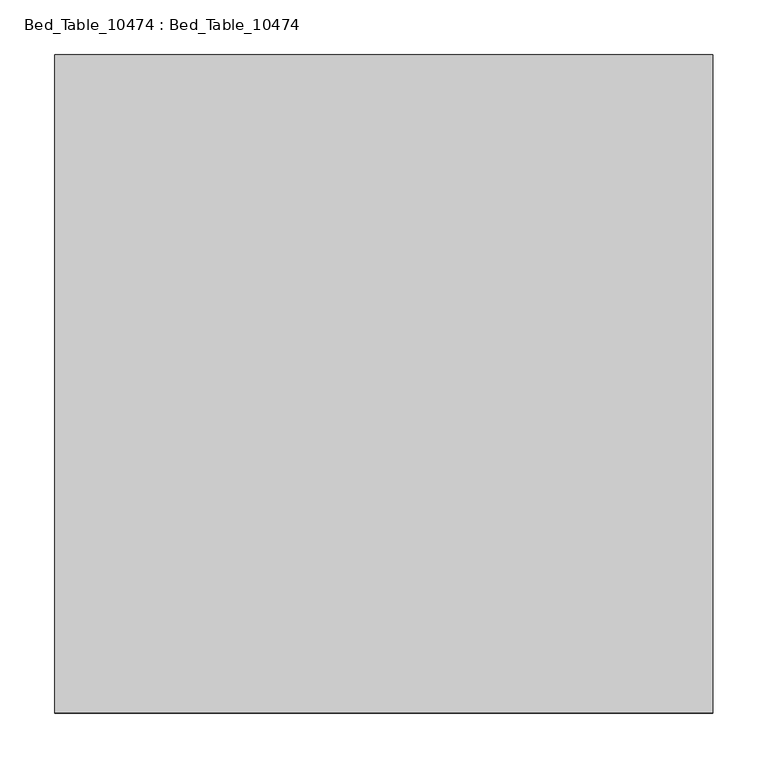
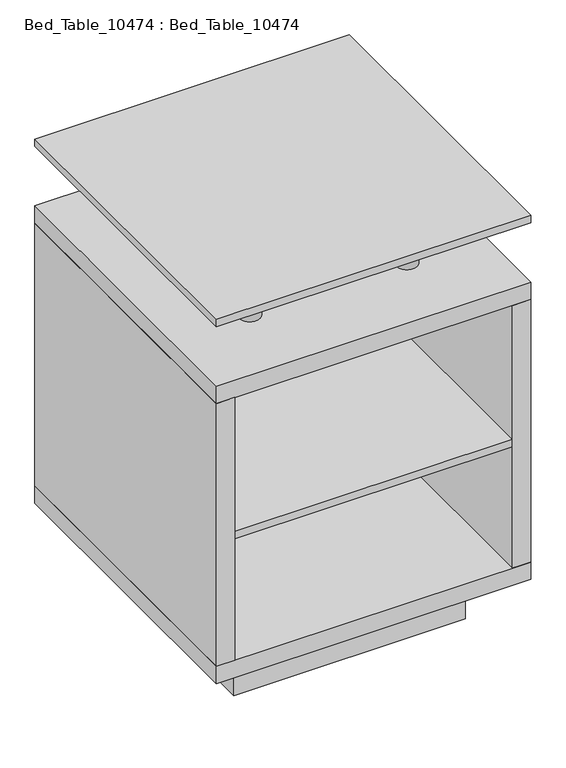
"""IFC4 building model written with IfcOpenShell, lengths in millimetres: furniture geometry, Bed_Table_10474 : Bed_Table_10474."""

from ifc_helpers import new_model, si_unit, point, frame, frame_2d, origin, origin_with_axes, place, context, project, spatial, polyline, circle_curve, trimmed, segment, composite_curve, outline, extrude, source, transform, mapped, element, save


def bed_table_10474_bed_table_10474_77ad9a9a(model_context):
    return source(origin(), model_context, "Body", "SweptSolid", [
        extrude(outline(polyline([(-265.0, 300.0), (-265.0, -300.0), (-300.0, -300.0), (-300.0, 300.0), (-265.0, 300.0)])), frame((0.0, 0.0, 135.0), z_axis=(0.0, 0.0, 1.0), x_axis=(1.0, 0.0, 0.0)), (0.0, 0.0, 1.0), 530.0),
        extrude(outline(polyline([(300.0, 300.0), (300.0, -300.0), (-300.0, -300.0), (-300.0, 300.0), (300.0, 300.0)])), frame((0.0, 0.0, 100.0), z_axis=(0.0, 0.0, 1.0), x_axis=(1.0, 0.0, 0.0)), (0.0, 0.0, 1.0), 35.0),
        extrude(outline(polyline([(300.0, 300.0), (300.0, -300.0), (-300.0, -300.0), (-300.0, 300.0), (300.0, 300.0)])), frame((0.0, 0.0, 665.0), z_axis=(0.0, 0.0, 1.0), x_axis=(1.0, 0.0, 0.0)), (0.0, 0.0, 1.0), 35.0),
        extrude(outline(polyline([(300.0, 300.0), (300.0, -300.0), (265.0, -300.0), (265.0, 300.0), (300.0, 300.0)])), frame((0.0, 0.0, 135.0), z_axis=(0.0, 0.0, 1.0), x_axis=(1.0, 0.0, 0.0)), (0.0, 0.0, 1.0), 530.0),
        extrude(outline(composite_curve([segment(trimmed(circle_curve(frame_2d((-150.0, 150.0)), 20.0), [point((-170.0, 150.0))], [point((-130.0, 150.0))], False, "CARTESIAN"), True, "CONTINUOUS"), segment(trimmed(circle_curve(frame_2d((-150.0, 150.0)), 20.0), [point((-130.0, 150.0))], [point((-170.0, 150.0))], False, "CARTESIAN"), True, "CONTINUOUS")], self_intersect=False)), frame((0.0, 0.0, 700.0), z_axis=(0.0, 0.0, 1.0), x_axis=(1.0, 0.0, 0.0)), (0.0, 0.0, 1.0), 120.0),
        extrude(outline(composite_curve([segment(trimmed(circle_curve(frame_2d((150.0, 150.0)), 20.0), [point((130.0, 150.0))], [point((170.0, 150.0))], False, "CARTESIAN"), True, "CONTINUOUS"), segment(trimmed(circle_curve(frame_2d((150.0, 150.0)), 20.0), [point((170.0, 150.0))], [point((130.0, 150.0))], False, "CARTESIAN"), True, "CONTINUOUS")], self_intersect=False)), frame((0.0, 0.0, 700.0), z_axis=(0.0, 0.0, 1.0), x_axis=(1.0, 0.0, 0.0)), (0.0, 0.0, 1.0), 120.0),
        extrude(outline(composite_curve([segment(trimmed(circle_curve(frame_2d((-150.0, -150.0)), 20.0), [point((-170.0, -150.0))], [point((-130.0, -150.0))], False, "CARTESIAN"), True, "CONTINUOUS"), segment(trimmed(circle_curve(frame_2d((-150.0, -150.0)), 20.0), [point((-130.0, -150.0))], [point((-170.0, -150.0))], False, "CARTESIAN"), True, "CONTINUOUS")], self_intersect=False)), frame((0.0, 0.0, 700.0), z_axis=(0.0, 0.0, 1.0), x_axis=(1.0, 0.0, 0.0)), (0.0, 0.0, 1.0), 120.0),
        extrude(outline(composite_curve([segment(trimmed(circle_curve(frame_2d((150.0, -150.0)), 20.0), [point((130.0, -150.0))], [point((170.0, -150.0))], False, "CARTESIAN"), True, "CONTINUOUS"), segment(trimmed(circle_curve(frame_2d((150.0, -150.0)), 20.0), [point((170.0, -150.0))], [point((130.0, -150.0))], False, "CARTESIAN"), True, "CONTINUOUS")], self_intersect=False)), frame((0.0, 0.0, 700.0), z_axis=(0.0, 0.0, 1.0), x_axis=(1.0, 0.0, 0.0)), (0.0, 0.0, 1.0), 120.0),
        extrude(outline(polyline([(300.0, 300.0), (300.0, -300.0), (-300.0, -300.0), (-300.0, 300.0), (300.0, 300.0)])), frame((0.0, 0.0, 820.0), z_axis=(0.0, 0.0, 1.0), x_axis=(1.0, 0.0, 0.0)), (0.0, 0.0, 1.0), 15.0),
        extrude(outline(polyline([(265.0, 300.0), (265.0, -300.0), (-265.0, -300.0), (-265.0, 300.0), (265.0, 300.0)])), frame((0.0, 0.0, 380.0), z_axis=(0.0, 0.0, 1.0), x_axis=(1.0, 0.0, 0.0)), (0.0, 0.0, 1.0), 15.0),
        extrude(outline(composite_curve([segment(trimmed(circle_curve(frame_2d((-150.0, 150.0)), 20.0), [point((-170.0, 150.0))], [point((-130.0, 150.0))], False, "CARTESIAN"), True, "CONTINUOUS"), segment(trimmed(circle_curve(frame_2d((-150.0, 150.0)), 20.0), [point((-130.0, 150.0))], [point((-170.0, 150.0))], False, "CARTESIAN"), True, "CONTINUOUS")], self_intersect=False)), origin_with_axes(), (0.0, 0.0, 1.0), 100.0),
        extrude(outline(composite_curve([segment(trimmed(circle_curve(frame_2d((150.0, 150.0)), 20.0), [point((130.0, 150.0))], [point((170.0, 150.0))], False, "CARTESIAN"), True, "CONTINUOUS"), segment(trimmed(circle_curve(frame_2d((150.0, 150.0)), 20.0), [point((170.0, 150.0))], [point((130.0, 150.0))], False, "CARTESIAN"), True, "CONTINUOUS")], self_intersect=False)), origin_with_axes(), (0.0, 0.0, 1.0), 100.0),
        extrude(outline(composite_curve([segment(trimmed(circle_curve(frame_2d((-150.0, -150.0)), 20.0), [point((-170.0, -150.0))], [point((-130.0, -150.0))], False, "CARTESIAN"), True, "CONTINUOUS"), segment(trimmed(circle_curve(frame_2d((-150.0, -150.0)), 20.0), [point((-130.0, -150.0))], [point((-170.0, -150.0))], False, "CARTESIAN"), True, "CONTINUOUS")], self_intersect=False)), origin_with_axes(), (0.0, 0.0, 1.0), 100.0),
        extrude(outline(composite_curve([segment(trimmed(circle_curve(frame_2d((150.0, -150.0)), 20.0), [point((130.0, -150.0))], [point((170.0, -150.0))], False, "CARTESIAN"), True, "CONTINUOUS"), segment(trimmed(circle_curve(frame_2d((150.0, -150.0)), 20.0), [point((170.0, -150.0))], [point((130.0, -150.0))], False, "CARTESIAN"), True, "CONTINUOUS")], self_intersect=False)), origin_with_axes(), (0.0, 0.0, 1.0), 100.0),
        extrude(outline(polyline([(-220.7106781, 220.7106781), (220.7106781, 220.7106781), (220.7106781, -220.7106781), (-220.7106781, -220.7106781), (-220.7106781, 220.7106781)]), holes=[polyline([(-210.7106781, 210.7106781), (-210.7106781, -210.7106781), (210.7106781, -210.7106781), (210.7106781, 210.7106781), (-210.7106781, 210.7106781)])]), origin_with_axes(), (0.0, 0.0, 1.0), 100.0),
    ])


if __name__ == "__main__":
    model = new_model("IFC4")
    model_context = context("Model", 3, world=origin())
    ifc_project = project(units=[si_unit("LENGTHUNIT", "METRE", prefix="MILLI")], contexts=[model_context])
    site = spatial("IfcSite", under=ifc_project)
    building = spatial("IfcBuilding", under=site)
    placement = place(None, origin())
    bed_table_10474_bed_table_10474_shape = bed_table_10474_bed_table_10474_77ad9a9a(model_context)
    element("IfcFurniture", 1, ObjectType="Bed_Table_10474 : Bed_Table_10474", at=placement, inside=building, context=model_context, shape_type="MappedRepresentation", body=[
        mapped(bed_table_10474_bed_table_10474_shape, transform((0.0, 0.0, 0.0), x_axis=(1.0, 0.0, 0.0), y_axis=(0.0, 1.0, 0.0), z_axis=(0.0, 0.0, 1.0))),
    ])
    save(model, "model.ifc")

# Revit data of these elements
# Type "Bed_Table_10474 : Bed_Table_10474"
#   myf = ""
#   Default Elevation = 0
# Element 1 (IfcFurniture, "Bed_Table_10474 : Bed_Table_10474")
#   Materials on its faces: "metal table", "madera", "glass table"
# Materials
#   "metal table": class "Metal", colour RGB 168 168 168, transparency 0
#   "madera": class "Wood", colour RGB 191 159 105, transparency 0
#   "glass table": class "Glass", colour RGB 229 191 0, transparency 0.95
